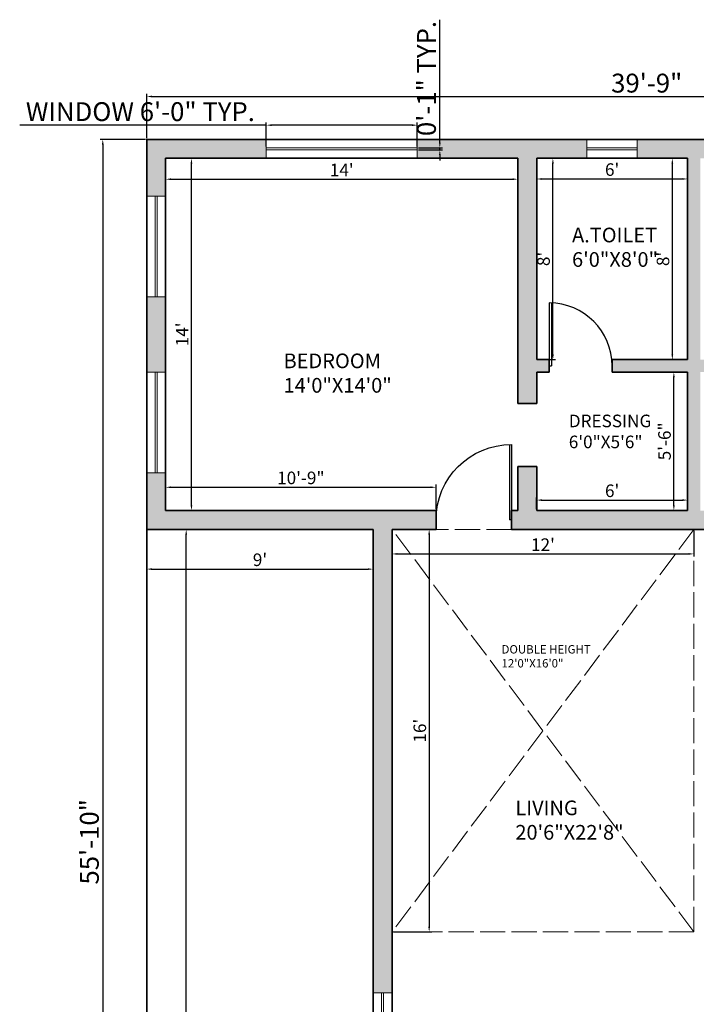
# Model space of a CAD drawing. Units: inches. Extents: x 4606 to 5879, y 1332 to 2209.
# Tile 6 of 7: x 5284 to 5607, y 1669 to 2138. Entities that reach past the tile are written whole.
import ezdxf

# ---------------------------------------------------------------- set-up
doc = ezdxf.new("R2010")
doc.units = ezdxf.units.IN
doc.linetypes.add('ACAD_ISO02W100', pattern=[15, 12, -3])
for name, color, linetype, lineweight in [('A-ANNO-DIMS', 2, 'Continuous', 18), ('A-AREA-IDEN', 7, 'Continuous', 18), ('A-DOOR', 4, 'Continuous', 25), ('A-FLOR-OVHD', 8, 'ACAD_ISO02W100', 13), ('A-WALL', 7, 'Continuous', 35), ('A-WALL-PATT', 252, 'Continuous', 13), ('window', 130, 'Continuous', 18)]:
    doc.layers.add(name, color=color, linetype=linetype, lineweight=lineweight)
doc.styles.get("Standard").update_dxf_attribs({"font": 'arial.ttf'})
doc.dimstyles.new('ISO-25', dxfattribs={"dimtxt": 9, "dimasz": 2.5, "dimexe": 1.25, "dimexo": 0.625, "dimtad": 1, "dimlunit": 3, "dimtxsty": 'Standard', "dimcen": 2.5, "dimadec": 0, "dimazin": 0, "dimtfac": 1, "dimtmove": 0, "dimatfit": 3, "dimfxl": 1, "dimarcsym": 0})

# ---------------------------------------------------------------- blocks, each defined once
blk = doc.blocks.new('*D25')
at = {"layer": 'A-ANNO-DIMS', "color": 0, "lineweight": -2, "transparency": 16777216}
for p, q in [((5344.86, 2081.86), (5344.86, 2102.96)), ((5347.36, 2101.71), (5819.36, 2101.71)), ((5821.86, 2081.86), (5821.86, 2102.96))]:
    blk.add_line(p, q, dxfattribs=at)
at = {"layer": 'A-ANNO-DIMS', "color": 0, "transparency": 16777216}
for points in [[(5347.36, 2102.13), (5347.36, 2101.29), (5344.86, 2101.71)], [(5819.36, 2102.13), (5819.36, 2101.29), (5821.86, 2101.71)]]:
    blk.add_solid(points, dxfattribs=at)
at = {"layer": 'Defpoints', "color": 0, "transparency": 16777216}
for p in [(5821.86, 2101.71), (5344.86, 2081.24), (5821.86, 2081.24)]:
    blk.add_point(p, dxfattribs=at)
at = {"layer": 'A-ANNO-DIMS', "color": 0, "transparency": 16777216, "insert": (5583.36, 2106.93), "char_height": 9, "attachment_point": 5}
blk.add_mtext('39\'-9"', dxfattribs=at)
blk = doc.blocks.new('D1')
for p, q in [((0, 36), (0, 0)), ((1, 36), (1, 0)), ((0, 0), (1, 0))]:
    blk.add_line(p, q)
blk.add_arc((0, 0), 36, 0, 90)
blk = doc.blocks.new('D2')
for p, q in [((0, 30), (0, 0)), ((1, 30), (1, 0)), ((0, 0), (1, 0))]:
    blk.add_line(p, q)
blk.add_arc((0, 0), 30, 0, 90)
blk = doc.blocks.new('*D26')
at = {"layer": 'A-ANNO-DIMS', "color": 0, "lineweight": -2, "transparency": 16777216}
for p, q in [((5344.24, 2081.24), (5322.61, 2081.24)), ((5323.86, 2078.74), (5323.86, 1413.74)), ((5344.24, 1411.24), (5322.61, 1411.24))]:
    blk.add_line(p, q, dxfattribs=at)
at = {"layer": 'A-ANNO-DIMS', "color": 0, "transparency": 16777216}
for points in [[(5323.44, 2078.74), (5324.28, 2078.74), (5323.86, 2081.24)], [(5323.44, 1413.74), (5324.28, 1413.74), (5323.86, 1411.24)]]:
    blk.add_solid(points, dxfattribs=at)
at = {"layer": 'Defpoints', "color": 0, "transparency": 16777216}
for p in [(5344.86, 2081.24), (5323.86, 1411.24), (5344.86, 1411.24)]:
    blk.add_point(p, dxfattribs=at)
at = {"layer": 'A-ANNO-DIMS', "color": 0, "transparency": 16777216, "insert": (5318.64, 1746.24), "char_height": 9, "attachment_point": 5, "rotation": 90}
blk.add_mtext('55\'-10"', dxfattribs=at)
blk = doc.blocks.new('*D27')
at = {"layer": 'A-ANNO-DIMS', "color": 0, "lineweight": -2, "transparency": 16777216}
for p, q in [((5353.86, 2071.61), (5353.86, 2061.02)), ((5521.86, 2071.61), (5521.86, 2061.02)), ((5356.36, 2062.27), (5519.36, 2062.27))]:
    blk.add_line(p, q, dxfattribs=at)
at = {"layer": 'A-ANNO-DIMS', "color": 0, "transparency": 16777216}
for points in [[(5356.36, 2062.69), (5356.36, 2061.85), (5353.86, 2062.27)], [(5519.36, 2062.69), (5519.36, 2061.85), (5521.86, 2062.27)]]:
    blk.add_solid(points, dxfattribs=at)
at = {"layer": 'Defpoints', "color": 0, "transparency": 16777216}
for p in [(5353.86, 2072.24), (5521.86, 2072.24), (5521.86, 2062.27)]:
    blk.add_point(p, dxfattribs=at)
at = {"layer": 'A-ANNO-DIMS', "color": 0, "transparency": 16777216, "insert": (5437.86, 2065.91), "char_height": 6, "attachment_point": 5}
blk.add_mtext("14'", dxfattribs=at)
blk = doc.blocks.new('*D28')
at = {"layer": 'A-ANNO-DIMS', "color": 0, "lineweight": -2, "transparency": 16777216}
for p, q in [((5354.49, 2072.24), (5367.42, 2072.24)), ((5366.17, 1906.74), (5366.17, 2069.74)), ((5354.49, 1904.24), (5367.42, 1904.24))]:
    blk.add_line(p, q, dxfattribs=at)
at = {"layer": 'A-ANNO-DIMS', "color": 0, "transparency": 16777216}
for points in [[(5365.76, 2069.74), (5366.59, 2069.74), (5366.17, 2072.24)], [(5365.76, 1906.74), (5366.59, 1906.74), (5366.17, 1904.24)]]:
    blk.add_solid(points, dxfattribs=at)
at = {"layer": 'Defpoints', "color": 0, "transparency": 16777216}
for p in [(5353.86, 2072.24), (5366.17, 2072.24), (5353.86, 1904.24)]:
    blk.add_point(p, dxfattribs=at)
at = {"layer": 'A-ANNO-DIMS', "color": 0, "transparency": 16777216, "insert": (5362.53, 1988.24), "char_height": 6, "attachment_point": 5, "rotation": 90}
blk.add_mtext("14'", dxfattribs=at)
blk = doc.blocks.new('*D31')
at = {"layer": 'A-ANNO-DIMS', "color": 0, "lineweight": -2, "transparency": 16777216}
for p, q in [((5530.86, 2071.61), (5530.86, 2061.13)), ((5602.86, 2071.61), (5602.86, 2061.13)), ((5533.36, 2062.38), (5600.36, 2062.38))]:
    blk.add_line(p, q, dxfattribs=at)
at = {"layer": 'A-ANNO-DIMS', "color": 0, "transparency": 16777216}
for points in [[(5533.36, 2062.79), (5533.36, 2061.96), (5530.86, 2062.38)], [(5600.36, 2062.79), (5600.36, 2061.96), (5602.86, 2062.38)]]:
    blk.add_solid(points, dxfattribs=at)
at = {"layer": 'Defpoints', "color": 0, "transparency": 16777216}
for p in [(5530.86, 2072.24), (5602.86, 2072.24), (5602.86, 2062.38)]:
    blk.add_point(p, dxfattribs=at)
at = {"layer": 'A-ANNO-DIMS', "color": 0, "transparency": 16777216, "insert": (5566.86, 2066.07), "char_height": 6, "attachment_point": 5}
blk.add_mtext("6'", dxfattribs=at)
blk = doc.blocks.new('*D32')
at = {"layer": 'A-ANNO-DIMS', "color": 0, "lineweight": -2, "transparency": 16777216}
for p, q in [((5602.24, 2072.24), (5594.34, 2072.24)), ((5595.59, 1978.74), (5595.59, 2069.74)), ((5602.24, 1976.24), (5594.34, 1976.24))]:
    blk.add_line(p, q, dxfattribs=at)
at = {"layer": 'A-ANNO-DIMS', "color": 0, "transparency": 16777216}
for points in [[(5595.17, 2069.74), (5596, 2069.74), (5595.59, 2072.24)], [(5595.17, 1978.74), (5596, 1978.74), (5595.59, 1976.24)]]:
    blk.add_solid(points, dxfattribs=at)
at = {"layer": 'Defpoints', "color": 0, "transparency": 16777216}
for p in [(5595.59, 2072.24), (5602.86, 2072.24), (5602.86, 1976.24)]:
    blk.add_point(p, dxfattribs=at)
at = {"layer": 'A-ANNO-DIMS', "color": 0, "transparency": 16777216, "insert": (5591.9, 2024.24), "char_height": 6, "attachment_point": 5, "rotation": 90}
blk.add_mtext("8'", dxfattribs=at)
blk = doc.blocks.new('*D35')
at = {"layer": 'A-ANNO-DIMS', "color": 0, "lineweight": -2, "transparency": 16777216}
for p, q in [((5531.49, 2072.24), (5539.85, 2072.24)), ((5538.6, 1978.74), (5538.6, 2069.74)), ((5531.49, 1976.24), (5539.85, 1976.24))]:
    blk.add_line(p, q, dxfattribs=at)
at = {"layer": 'A-ANNO-DIMS', "color": 0, "transparency": 16777216}
for points in [[(5538.18, 2069.74), (5539.02, 2069.74), (5538.6, 2072.24)], [(5538.18, 1978.74), (5539.02, 1978.74), (5538.6, 1976.24)]]:
    blk.add_solid(points, dxfattribs=at)
at = {"layer": 'Defpoints', "color": 0, "transparency": 16777216}
for p in [(5530.86, 2072.24), (5538.6, 2072.24), (5530.86, 1976.24)]:
    blk.add_point(p, dxfattribs=at)
at = {"layer": 'A-ANNO-DIMS', "color": 0, "transparency": 16777216, "insert": (5534.91, 2024.24), "char_height": 6, "attachment_point": 5, "rotation": 90}
blk.add_mtext("8'", dxfattribs=at)
blk = doc.blocks.new('*D36')
at = {"layer": 'A-ANNO-DIMS', "color": 0, "lineweight": -2, "transparency": 16777216}
for p, q in [((5353.86, 1904.86), (5353.86, 1916.59)), ((5482.86, 1904.86), (5482.86, 1916.59)), ((5356.36, 1915.34), (5480.36, 1915.34))]:
    blk.add_line(p, q, dxfattribs=at)
at = {"layer": 'A-ANNO-DIMS', "color": 0, "transparency": 16777216}
for points in [[(5356.36, 1915.76), (5356.36, 1914.92), (5353.86, 1915.34)], [(5480.36, 1915.76), (5480.36, 1914.92), (5482.86, 1915.34)]]:
    blk.add_solid(points, dxfattribs=at)
at = {"layer": 'Defpoints', "color": 0, "transparency": 16777216}
for p in [(5482.86, 1915.34), (5353.86, 1904.24), (5482.86, 1904.24)]:
    blk.add_point(p, dxfattribs=at)
at = {"layer": 'A-ANNO-DIMS', "color": 0, "transparency": 16777216, "insert": (5418.36, 1919.03), "char_height": 6, "attachment_point": 5}
blk.add_mtext('10\'-9"', dxfattribs=at)
blk = doc.blocks.new('*D37')
at = {"layer": 'A-ANNO-DIMS', "color": 0, "lineweight": -2, "transparency": 16777216}
for p, q in [((5530.86, 1904.86), (5530.86, 1910.46)), ((5533.36, 1909.21), (5600.36, 1909.21)), ((5602.86, 1904.86), (5602.86, 1910.46))]:
    blk.add_line(p, q, dxfattribs=at)
at = {"layer": 'A-ANNO-DIMS', "color": 0, "transparency": 16777216}
for points in [[(5533.36, 1909.63), (5533.36, 1908.8), (5530.86, 1909.21)], [(5600.36, 1909.63), (5600.36, 1908.8), (5602.86, 1909.21)]]:
    blk.add_solid(points, dxfattribs=at)
at = {"layer": 'Defpoints', "color": 0, "transparency": 16777216}
for p in [(5602.86, 1909.21), (5530.86, 1904.24), (5602.86, 1904.24)]:
    blk.add_point(p, dxfattribs=at)
at = {"layer": 'A-ANNO-DIMS', "color": 0, "transparency": 16777216, "insert": (5566.86, 1912.9), "char_height": 6, "attachment_point": 5}
blk.add_mtext("6'", dxfattribs=at)
blk = doc.blocks.new('*D38')
at = {"layer": 'A-ANNO-DIMS', "color": 0, "lineweight": -2, "transparency": 16777216}
for p, q in [((5602.24, 1970.24), (5595.05, 1970.24)), ((5596.3, 1906.74), (5596.3, 1967.74)), ((5602.24, 1904.24), (5595.05, 1904.24))]:
    blk.add_line(p, q, dxfattribs=at)
at = {"layer": 'A-ANNO-DIMS', "color": 0, "transparency": 16777216}
for points in [[(5595.89, 1967.74), (5596.72, 1967.74), (5596.3, 1970.24)], [(5595.89, 1906.74), (5596.72, 1906.74), (5596.3, 1904.24)]]:
    blk.add_solid(points, dxfattribs=at)
at = {"layer": 'Defpoints', "color": 0, "transparency": 16777216}
for p in [(5596.3, 1970.24), (5602.86, 1970.24), (5602.86, 1904.24)]:
    blk.add_point(p, dxfattribs=at)
at = {"layer": 'A-ANNO-DIMS', "color": 0, "transparency": 16777216, "insert": (5592.62, 1937.24), "char_height": 6, "attachment_point": 5, "rotation": 90}
blk.add_mtext('5\'-6"', dxfattribs=at)
blk = doc.blocks.new('*D57')
at = {"layer": 'A-ANNO-DIMS', "color": 0, "lineweight": -2, "transparency": 16777216}
for p, q in [((5345.49, 1895.24), (5364.92, 1895.24)), ((5363.67, 1413.74), (5363.67, 1892.74)), ((5345.49, 1411.24), (5364.92, 1411.24))]:
    blk.add_line(p, q, dxfattribs=at)
at = {"layer": 'A-ANNO-DIMS', "color": 0, "transparency": 16777216}
for points in [[(5363.25, 1892.74), (5364.08, 1892.74), (5363.67, 1895.24)], [(5363.25, 1413.74), (5364.08, 1413.74), (5363.67, 1411.24)]]:
    blk.add_solid(points, dxfattribs=at)
at = {"layer": 'Defpoints', "color": 0, "transparency": 16777216}
for p in [(5344.86, 1895.24), (5363.67, 1895.24), (5344.86, 1411.24)]:
    blk.add_point(p, dxfattribs=at)
at = {"layer": 'A-ANNO-DIMS', "color": 0, "transparency": 16777216, "insert": (5359.98, 1653.24), "char_height": 6, "attachment_point": 5, "rotation": 90}
blk.add_mtext('40\'-4"', dxfattribs=at)
blk = doc.blocks.new('*D58')
at = {"layer": 'A-ANNO-DIMS', "color": 0, "lineweight": -2, "transparency": 16777216}
for p, q in [((5344.86, 1894.61), (5344.86, 1875.05)), ((5452.86, 1894.61), (5452.86, 1875.05)), ((5347.36, 1876.3), (5450.36, 1876.3))]:
    blk.add_line(p, q, dxfattribs=at)
at = {"layer": 'A-ANNO-DIMS', "color": 0, "transparency": 16777216}
for points in [[(5347.36, 1876.72), (5347.36, 1875.89), (5344.86, 1876.3)], [(5450.36, 1876.72), (5450.36, 1875.89), (5452.86, 1876.3)]]:
    blk.add_solid(points, dxfattribs=at)
at = {"layer": 'Defpoints', "color": 0, "transparency": 16777216}
for p in [(5344.86, 1895.24), (5452.86, 1895.24), (5452.86, 1876.3)]:
    blk.add_point(p, dxfattribs=at)
at = {"layer": 'A-ANNO-DIMS', "color": 0, "transparency": 16777216, "insert": (5398.86, 1879.99), "char_height": 6, "attachment_point": 5}
blk.add_mtext("9'", dxfattribs=at)
blk = doc.blocks.new('*D59')
at = {"layer": 'A-ANNO-DIMS', "color": 0, "lineweight": -2, "transparency": 16777216}
for p, q in [((5461.86, 1894.61), (5461.86, 1882.3)), ((5605.86, 1894.61), (5605.86, 1882.3)), ((5464.36, 1883.55), (5603.36, 1883.55))]:
    blk.add_line(p, q, dxfattribs=at)
at = {"layer": 'A-ANNO-DIMS', "color": 0, "transparency": 16777216}
for points in [[(5464.36, 1883.96), (5464.36, 1883.13), (5461.86, 1883.55)], [(5603.36, 1883.96), (5603.36, 1883.13), (5605.86, 1883.55)]]:
    blk.add_solid(points, dxfattribs=at)
at = {"layer": 'Defpoints', "color": 0, "transparency": 16777216}
for p in [(5461.86, 1895.24), (5605.86, 1895.24), (5605.86, 1883.55)]:
    blk.add_point(p, dxfattribs=at)
at = {"layer": 'A-ANNO-DIMS', "color": 0, "transparency": 16777216, "insert": (5533.86, 1887.19), "char_height": 6, "attachment_point": 5}
blk.add_mtext("12'", dxfattribs=at)
blk = doc.blocks.new('*D60')
at = {"layer": 'A-ANNO-DIMS', "color": 0, "lineweight": -2, "transparency": 16777216}
for p, q in [((5462.49, 1895.24), (5480.83, 1895.24)), ((5479.58, 1892.74), (5479.58, 1705.74)), ((5462.49, 1703.24), (5480.83, 1703.24))]:
    blk.add_line(p, q, dxfattribs=at)
at = {"layer": 'A-ANNO-DIMS', "color": 0, "transparency": 16777216}
for points in [[(5479.16, 1892.74), (5480, 1892.74), (5479.58, 1895.24)], [(5479.16, 1705.74), (5480, 1705.74), (5479.58, 1703.24)]]:
    blk.add_solid(points, dxfattribs=at)
at = {"layer": 'Defpoints', "color": 0, "transparency": 16777216}
for p in [(5461.86, 1895.24), (5461.86, 1703.24), (5479.58, 1703.24)]:
    blk.add_point(p, dxfattribs=at)
at = {"layer": 'A-ANNO-DIMS', "color": 0, "transparency": 16777216, "insert": (5475.89, 1799.24), "char_height": 6, "attachment_point": 5, "rotation": 90}
blk.add_mtext("16'", dxfattribs=at)
blk = doc.blocks.new('GLAZING-72IN')
for p, q in [((0, 0), (0, 72)), ((1, 0), (1, 72))]:
    blk.add_line(p, q)
blk = doc.blocks.new('GLAZING-24IN')
for p, q in [((0, 0), (0, 24)), ((1, 0), (1, 24))]:
    blk.add_line(p, q)
blk = doc.blocks.new('GLAZING-48IN')
for p, q in [((0, 0), (0, 48)), ((1, 0), (1, 48))]:
    blk.add_line(p, q)
blk = doc.blocks.new('*D69')
at = {"layer": 'A-ANNO-DIMS', "color": 0, "lineweight": -2, "transparency": 16777216}
for p, q in [((5401.86, 2088.04), (5284.23, 2088.04)), ((5401.86, 2077.86), (5401.86, 2089.29)), ((5471.36, 2088.04), (5404.36, 2088.04)), ((5473.86, 2077.86), (5473.86, 2089.29))]:
    blk.add_line(p, q, dxfattribs=at)
at = {"layer": 'A-ANNO-DIMS', "color": 0, "transparency": 16777216}
for points in [[(5404.36, 2088.46), (5404.36, 2087.62), (5401.86, 2088.04)], [(5471.36, 2088.46), (5471.36, 2087.62), (5473.86, 2088.04)]]:
    blk.add_solid(points, dxfattribs=at)
at = {"layer": 'Defpoints', "color": 0, "transparency": 16777216}
for p in [(5401.86, 2088.04), (5401.86, 2077.24), (5473.86, 2077.24)]:
    blk.add_point(p, dxfattribs=at)
at = {"layer": 'A-ANNO-DIMS', "color": 0, "transparency": 16777216, "insert": (5341.8, 2093.32), "char_height": 9, "attachment_point": 5}
blk.add_mtext('WINDOW 6\'-0" TYP.', dxfattribs=at)
blk = doc.blocks.new('*D70')
at = {"layer": 'A-ANNO-DIMS', "color": 0, "lineweight": -2, "transparency": 16777216}
for p, q in [((5484.66, 2079.74), (5484.66, 2138.35)), ((5474.49, 2077.24), (5485.91, 2077.24)), ((5474.49, 2076.24), (5485.91, 2076.24)), ((5484.66, 2076.24), (5484.66, 2077.24)), ((5484.66, 2073.74), (5484.66, 2071.24))]:
    blk.add_line(p, q, dxfattribs=at)
at = {"layer": 'A-ANNO-DIMS', "color": 0, "transparency": 16777216}
for points in [[(5484.25, 2079.74), (5485.08, 2079.74), (5484.66, 2077.24)], [(5484.25, 2073.74), (5485.08, 2073.74), (5484.66, 2076.24)]]:
    blk.add_solid(points, dxfattribs=at)
at = {"layer": 'Defpoints', "color": 0, "transparency": 16777216}
for p in [(5473.86, 2077.24), (5473.86, 2076.24), (5484.66, 2077.24)]:
    blk.add_point(p, dxfattribs=at)
at = {"layer": 'A-ANNO-DIMS', "color": 0, "transparency": 16777216, "insert": (5479.44, 2110.29), "char_height": 9, "attachment_point": 5, "rotation": 90}
blk.add_mtext('0\'-1" TYP.', dxfattribs=at)
blk = doc.blocks.new('*D79')
at = {"layer": 'A-ANNO-DIMS', "color": 0, "lineweight": -2, "transparency": 16777216}
for p, q in [((5636.76, 1602.24), (5636.76, 1721.18)), ((5631.99, 1602.24), (5638.01, 1602.24)), ((5636.76, 1568.74), (5636.76, 1599.74)), ((5631.99, 1566.24), (5638.01, 1566.24))]:
    blk.add_line(p, q, dxfattribs=at)
at = {"layer": 'A-ANNO-DIMS', "color": 0, "transparency": 16777216}
for points in [[(5636.35, 1599.74), (5637.18, 1599.74), (5636.76, 1602.24)], [(5636.35, 1568.74), (5637.18, 1568.74), (5636.76, 1566.24)]]:
    blk.add_solid(points, dxfattribs=at)
at = {"layer": 'Defpoints', "color": 0, "transparency": 16777216}
for p in [(5631.36, 1602.24), (5636.76, 1602.24), (5631.36, 1566.24)]:
    blk.add_point(p, dxfattribs=at)
at = {"layer": 'A-ANNO-DIMS', "color": 0, "transparency": 16777216, "insert": (5631.48, 1662.96), "char_height": 9, "attachment_point": 5, "rotation": 90}
blk.add_mtext('DOOR D3 3\'-0" TYP.', dxfattribs=at)

msp = doc.modelspace()

# ---------------------------------------------------------------- hatches: boundary and pattern name
at = {"layer": 'A-WALL-PATT', "transparency": 33554687}
h = msp.add_hatch(color=256, dxfattribs=at)
h.dxf.hatch_style = 1
h.paths.add_polyline_path([(5635.864, 1512.239), (5626.864, 1512.239), (5626.864, 1420.239), (5566.864, 1420.239), (5566.864, 1545.239), (5626.864, 1545.239), (5626.864, 1542.239), (5631.364, 1542.239), (5635.864, 1542.239), (5635.864, 1566.239), (5626.864, 1566.239), (5626.864, 1554.239), (5566.864, 1554.239), (5566.864, 1614.239), (5626.864, 1614.239), (5626.864, 1602.239), (5631.364, 1602.239), (5635.864, 1602.239), (5635.864, 1623.239), (5512.864, 1623.239), (5512.864, 1614.239), (5557.864, 1614.239), (5557.864, 1554.239), (5512.864, 1554.239), (5512.864, 1549.739), (5512.864, 1545.239), (5557.864, 1545.239), (5557.864, 1411.239), (5683.864, 1411.239), (5683.864, 1420.239), (5635.864, 1420.239)])
h.paths.add_polyline_path([(5788.864, 1446.239), (5779.864, 1446.239), (5779.864, 1420.239), (5731.864, 1420.239), (5731.864, 1411.239), (5788.864, 1411.239)])
h.paths.add_polyline_path([(5788.864, 1512.239), (5779.864, 1512.239), (5779.864, 1494.239), (5788.864, 1494.239)])
h.paths.add_polyline_path([(5788.864, 1591.739), (5779.864, 1591.739), (5779.864, 1542.239), (5788.864, 1542.239)])
h.paths.add_polyline_path([(5821.864, 1691.239), (5812.864, 1691.239), (5812.864, 1673.239), (5716.864, 1673.239), (5716.864, 1676.239), (5712.364, 1676.239), (5707.864, 1676.239), (5707.864, 1673.239), (5689.864, 1673.239), (5689.864, 1664.239), (5779.864, 1664.239), (5779.864, 1639.739), (5788.864, 1639.739), (5788.864, 1664.239), (5821.864, 1664.239)])
h.paths.add_polyline_path([(5821.864, 1823.239), (5812.864, 1823.239), (5812.864, 1799.239), (5714.864, 1799.239), (5714.864, 1790.239), (5743.864, 1790.239), (5743.864, 1784.239), (5752.864, 1784.239), (5752.864, 1790.239), (5812.864, 1790.239), (5812.864, 1742.239), (5752.864, 1742.239), (5752.864, 1748.239), (5743.864, 1748.239), (5743.864, 1742.239), (5707.864, 1742.239), (5707.864, 1706.239), (5716.864, 1706.239), (5716.864, 1733.239), (5812.864, 1733.239), (5812.864, 1715.239), (5821.864, 1715.239)])
h.paths.add_polyline_path([(5821.864, 1928.239), (5812.864, 1928.239), (5812.864, 1904.239), (5713.864, 1904.239), (5713.864, 1895.239), (5812.864, 1895.239), (5812.864, 1871.239), (5821.864, 1871.239)])
h.paths.add_polyline_path([(5821.864, 2006.239), (5812.864, 2006.239), (5812.864, 1976.239), (5821.864, 1976.239)])
h.paths.add_polyline_path([(5821.864, 2081.239), (5779.864, 2081.239), (5779.864, 2072.239), (5812.864, 2072.239), (5812.864, 2054.239), (5821.864, 2054.239)])
h.paths.add_polyline_path([(5707.864, 2081.239), (5650.864, 2081.239), (5650.864, 2072.239), (5668.864, 2072.239), (5668.864, 1976.239), (5662.864, 1976.239), (5662.864, 1970.239), (5668.864, 1970.239), (5668.864, 1955.239), (5674.864, 1955.239), (5674.864, 2072.239), (5707.864, 2072.239)])
h.paths.add_polyline_path([(5626.864, 2081.239), (5578.864, 2081.239), (5578.864, 2072.239), (5602.864, 2072.239), (5602.864, 1976.239), (5566.864, 1976.239), (5566.864, 1970.239), (5602.864, 1970.239), (5602.864, 1904.239), (5530.864, 1904.239), (5530.864, 1925.239), (5521.864, 1925.239), (5521.864, 1904.239), (5518.864, 1904.239), (5518.864, 1895.239), (5605.864, 1895.239), (5677.864, 1895.239), (5677.864, 1904.239), (5674.864, 1904.239), (5674.864, 1925.239), (5668.864, 1925.239), (5668.864, 1904.239), (5608.864, 1904.239), (5608.864, 1970.239), (5632.864, 1970.239), (5632.864, 1976.239), (5608.864, 1976.239), (5608.864, 2072.239), (5626.864, 2072.239)])
h.paths.add_polyline_path([(5554.864, 2081.239), (5473.864, 2081.239), (5473.864, 2072.239), (5521.864, 2072.239), (5521.864, 1955.239), (5530.864, 1955.239), (5530.864, 1970.239), (5536.864, 1970.239), (5536.864, 1976.239), (5530.864, 1976.239), (5530.864, 2072.239), (5554.864, 2072.239)])
h.paths.add_polyline_path([(5401.864, 2081.239), (5344.864, 2081.239), (5344.864, 2054.239), (5353.864, 2054.239), (5353.864, 2072.239), (5401.864, 2072.239)])
h.paths.add_polyline_path([(5353.864, 2006.239), (5344.864, 2006.239), (5344.864, 1970.239), (5353.864, 1970.239)])
h.paths.add_polyline_path([(5482.864, 1904.239), (5353.864, 1904.239), (5353.864, 1922.239), (5344.864, 1922.239), (5344.864, 1895.239), (5452.864, 1895.239), (5452.864, 1674.239), (5461.864, 1674.239), (5461.864, 1895.239), (5482.864, 1895.239)])
h.paths.add_polyline_path([(5461.864, 1602.239), (5452.864, 1602.239), (5452.864, 1474.239), (5461.864, 1474.239), (5461.864, 1545.239), (5464.864, 1545.239), (5464.864, 1554.239), (5461.864, 1554.239)])

# ---------------------------------------------------------------- linework, layer by layer
at = {"layer": 'A-FLOR-OVHD'}
for p, q in [((5605.864, 1703.239), (5461.864, 1895.239)), ((5605.864, 1895.239), (5461.864, 1703.239))]:
    msp.add_line(p, q, dxfattribs=at)
msp.add_lwpolyline([(5461.864, 1895.239), (5605.864, 1895.239), (5605.864, 1703.239), (5461.864, 1703.239)], close=True, dxfattribs=at)
at = {"layer": 'A-WALL'}
for p, q in [((5521.864, 2072.239), (5353.864, 2072.239)), ((5353.864, 2072.239), (5353.864, 1904.239)), ((5521.864, 2072.239), (5521.864, 1955.239)), ((5602.864, 2072.239), (5530.864, 2072.239)), ((5530.864, 2072.239), (5530.864, 1976.239)), ((5602.864, 2072.239), (5602.864, 1976.239)), ((5536.864, 1976.239), (5530.864, 1976.239)), ((5536.864, 1976.239), (5536.864, 1970.239)), ((5602.864, 1976.239), (5566.864, 1976.239)), ((5566.864, 1976.239), (5566.864, 1970.239)), ((5536.864, 1970.239), (5530.864, 1970.239)), ((5530.864, 1970.239), (5530.864, 1955.239)), ((5602.864, 1970.239), (5566.864, 1970.239)), ((5602.864, 1970.239), (5602.864, 1904.239)), ((5530.864, 1955.239), (5521.864, 1955.239)), ((5530.864, 1925.239), (5521.864, 1925.239)), ((5521.864, 1925.239), (5521.864, 1904.239)), ((5530.864, 1925.239), (5530.864, 1904.239)), ((5482.864, 1904.239), (5353.864, 1904.239)), ((5482.864, 1904.239), (5482.864, 1895.239)), ((5521.864, 1904.239), (5518.864, 1904.239)), ((5518.864, 1904.239), (5518.864, 1895.239)), ((5602.864, 1904.239), (5530.864, 1904.239)), ((5452.864, 1895.239), (5344.864, 1895.239)), ((5452.864, 1895.239), (5452.864, 1474.239)), ((5482.864, 1895.239), (5461.864, 1895.239)), ((5461.864, 1895.239), (5461.864, 1554.239)), ((5677.864, 1895.239), (5518.864, 1895.239))]:
    msp.add_line(p, q, dxfattribs=at)
msp.add_lwpolyline([(5821.864, 1664.239), (5821.864, 2081.239), (5344.864, 2081.239), (5344.864, 1411.239), (5788.864, 1411.239)], dxfattribs=at)
at = {"layer": 'window'}
for p, q in [((5401.864, 2072.239), (5401.864, 2081.239)), ((5473.864, 2072.239), (5473.864, 2081.239)), ((5554.864, 2072.239), (5554.864, 2081.239)), ((5578.864, 2072.239), (5578.864, 2081.239)), ((5353.864, 2054.239), (5344.864, 2054.239)), ((5353.864, 2006.239), (5344.864, 2006.239)), ((5353.864, 1970.239), (5344.864, 1970.239)), ((5353.864, 1922.239), (5344.864, 1922.239)), ((5452.864, 1674.239), (5461.864, 1674.239))]:
    msp.add_line(p, q, dxfattribs=at)

# ---------------------------------------------------------------- block references
at = {"layer": 'A-DOOR'}
msp.add_blockref('D2', (5536.864, 1973.239), dxfattribs=at)
at = {"layer": 'A-DOOR', "xscale": -1}
msp.add_blockref('D1', (5518.864, 1899.739), dxfattribs=at)
at = {"layer": 'window'}
for name, p, rotation in [('GLAZING-72IN', (5473.864, 2076.239), 90.00000000000003), ('GLAZING-24IN', (5578.864, 2076.239), 89.99999999999984)]:
    msp.add_blockref(name, p, dxfattribs=dict(at, rotation=rotation))
for name, p in [('GLAZING-48IN', (5348.864, 2006.239)), ('GLAZING-48IN', (5348.864, 1922.239)), ('GLAZING-72IN', (5456.864, 1602.239))]:
    msp.add_blockref(name, p, dxfattribs=at)

# ---------------------------------------------------------------- texts
at = {"layer": 'A-AREA-IDEN', "attachment_point": 1}
for s, insert, char_height in [('{\\fTimes New Roman|b0|i0|c0|p18;A.TOILET\\P6\'0"X8\'0"}', (5547.738, 2039.149), 7), ('{\\fTimes New Roman|b0|i0|c0|p18;BEDROOM\\P14\'0"X14\'0"}', (5410.1, 1979.126), 7), ('{\\fTimes New Roman|b0|i0|c0|p18;DRESSING\\P6\'0"X5\'6"}', (5546.189, 1949.974), 6), ('{\\fTimes New Roman|b0|i0|c0|p18;DOUBLE HEIGHT\\P12\'0"X16\'0"}', (5514.112, 1840.052), 4), ('{\\fTimes New Roman|b0|i0|c0|p18;LIVING\\P20\'6"X22\'8"}', (5520.697, 1765.94), 7)]:
    msp.add_mtext_dynamic_manual_height_columns(s, width=80.30411, gutter_width=12.5, heights=[0], dxfattribs=dict(at, insert=insert, char_height=char_height))

# ---------------------------------------------------------------- dimensions: what is measured, and where the dimension line sits
at = {"layer": 'A-ANNO-DIMS'}
for base, p1, p2, angle, text, picture, middle in [((5484.664, 2077.239), (5473.864, 2076.239), (5473.864, 2077.239), 90, '<> TYP.', '*D70', (5479.444, 2110.294)), ((5401.864, 2088.039), (5473.864, 2077.239), (5401.864, 2077.239), 180, 'WINDOW <> TYP.', '*D69', (5341.796, 2093.32)), ((5636.764, 1602.239), (5631.364, 1566.239), (5631.364, 1602.239), 90, 'DOOR D3 <> TYP.', '*D79', (5631.48, 1662.958))]:
    dim = msp.add_linear_dim(base=base, p1=p1, p2=p2, angle=angle, text=text, dimstyle='ISO-25', override={"dimdec": 1, "dimlfac": 1, "dimrnd": 0, "dimzin": 1, "dimdsep": 46, "dimlunit": 4, "dimfrac": 2}, dxfattribs=at)
    dim.commit()
    dim.dimension.update_dxf_attribs({"geometry": picture, "text_midpoint": middle})
for base, p1, p2, override, picture, middle in [((5821.864, 2101.71), (5344.864, 2081.239), (5821.864, 2081.239), {"dimclrd": 0, "dimclre": 0, "dimclrt": 0}, '*D25', (5583.364, 2106.933)), ((5521.864, 2062.271), (5353.864, 2072.239), (5521.864, 2072.239), {"dimtxt": 6, "dimclrd": 0, "dimclre": 0, "dimclrt": 0}, '*D27', (5437.864, 2065.908)), ((5602.864, 2062.378), (5530.864, 2072.239), (5602.864, 2072.239), {"dimtxt": 6, "dimclrd": 0, "dimclre": 0, "dimclrt": 0}, '*D31', (5566.864, 2066.066)), ((5482.864, 1915.341), (5353.864, 1904.239), (5482.864, 1904.239), {"dimtxt": 6, "dimclrd": 0, "dimclre": 0, "dimclrt": 0}, '*D36', (5418.364, 1919.03)), ((5602.864, 1909.212), (5530.864, 1904.239), (5602.864, 1904.239), {"dimtxt": 6, "dimclrd": 0, "dimclre": 0, "dimclrt": 0}, '*D37', (5566.864, 1912.9)), ((5452.864, 1876.302), (5344.864, 1895.239), (5452.864, 1895.239), {"dimtxt": 6, "dimclrd": 0, "dimclre": 0, "dimclrt": 0}, '*D58', (5398.864, 1879.991)), ((5605.864, 1883.548), (5461.864, 1895.239), (5605.864, 1895.239), {"dimtxt": 6, "dimclrd": 0, "dimclre": 0, "dimclrt": 0}, '*D59', (5533.864, 1887.185))]:
    dim = msp.add_linear_dim(base=base, p1=p1, p2=p2, dimstyle='ISO-25', override=override, dxfattribs=at)
    dim.commit()
    dim.dimension.update_dxf_attribs({"geometry": picture, "text_midpoint": middle})
for base, p1, p2, angle, override, picture, middle in [((5323.86, 1411.239), (5344.864, 2081.239), (5344.864, 1411.239), 90, {"dimclrd": 0, "dimclre": 0, "dimclrt": 0}, '*D26', (5318.639, 1746.239)), ((5366.172, 2072.239), (5353.864, 1904.239), (5353.864, 2072.239), 270, {"dimtxt": 6, "dimclrd": 0, "dimclre": 0, "dimclrt": 0}, '*D28', (5362.534, 1988.239)), ((5538.6, 2072.239), (5530.864, 1976.239), (5530.864, 2072.239), 270, {"dimtxt": 6, "dimclrd": 0, "dimclre": 0, "dimclrt": 0}, '*D35', (5534.912, 2024.239)), ((5595.588, 2072.239), (5602.864, 1976.239), (5602.864, 2072.239), 270, {"dimtxt": 6, "dimclrd": 0, "dimclre": 0, "dimclrt": 0}, '*D32', (5591.9, 2024.239)), ((5596.304, 1970.239), (5602.864, 1904.239), (5602.864, 1970.239), 270, {"dimtxt": 6, "dimclrd": 0, "dimclre": 0, "dimclrt": 0}, '*D38', (5592.615, 1937.239)), ((5363.666, 1895.239), (5344.864, 1411.239), (5344.864, 1895.239), 90, {"dimtxt": 6, "dimclrd": 0, "dimclre": 0, "dimclrt": 0}, '*D57', (5359.977, 1653.239)), ((5479.581, 1703.239), (5461.864, 1895.239), (5461.864, 1703.239), 90, {"dimtxt": 6, "dimclrd": 0, "dimclre": 0, "dimclrt": 0}, '*D60', (5475.893, 1799.239))]:
    dim = msp.add_linear_dim(base=base, p1=p1, p2=p2, angle=angle, dimstyle='ISO-25', override=override, dxfattribs=at)
    dim.commit()
    dim.dimension.update_dxf_attribs({"geometry": picture, "text_midpoint": middle})

doc.saveas('drawing.dxf')
